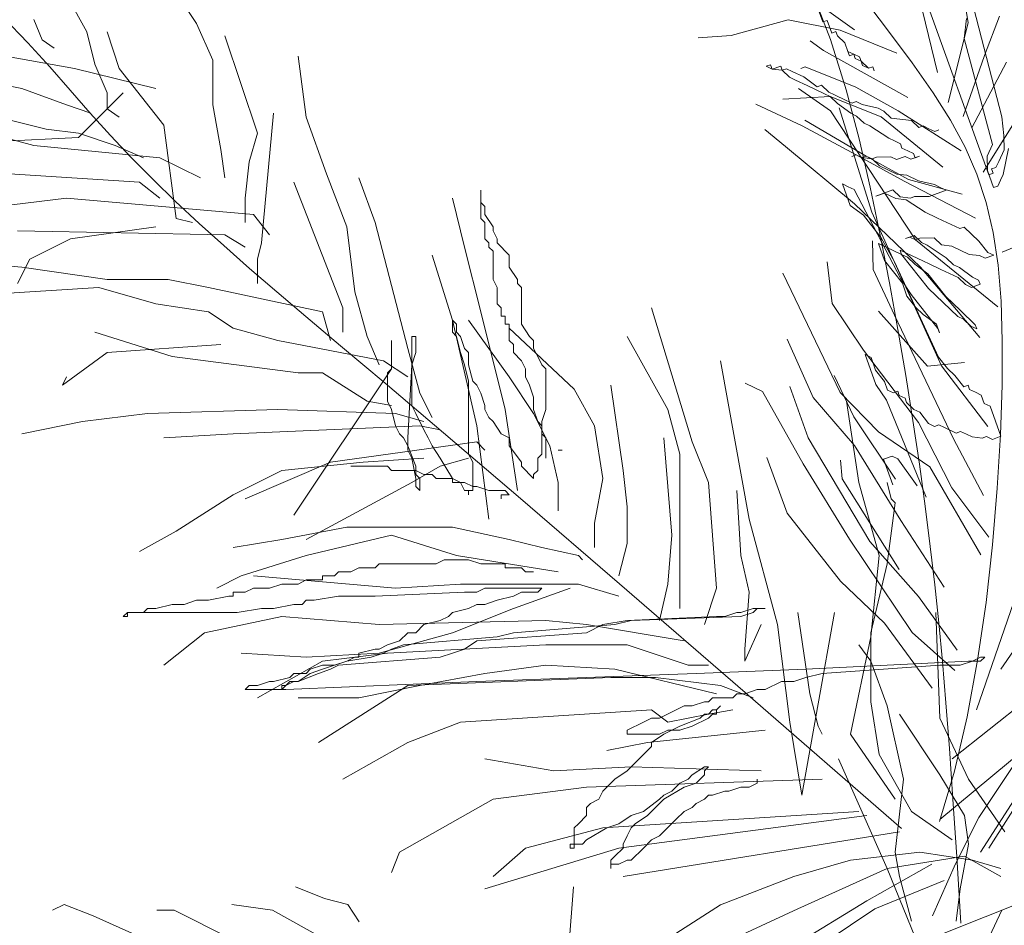
# Model space of a CAD drawing. Units: millimetres. Extents: x 595116 to 630915, y 909473 to 920225.
# Tile 87 of 134: x 629714.705 to 629720.901, y 919275.684 to 919281.384. Entities that reach past the tile are written whole.
import ezdxf

# ---------------------------------------------------------------- set-up
doc = ezdxf.new("R2010")
doc.units = ezdxf.units.MM
doc.layers.add('Dimension', color=3, linetype='Continuous', lineweight=18)
doc.layers.add('L-PLNT', color=85, linetype='Continuous', lineweight=13)
doc.styles.get("Standard").update_dxf_attribs({"font": 'arial.ttf'})
doc.dimstyles.new('ISO-25', dxfattribs={"dimtxt": 9, "dimasz": 6, "dimexe": 1.25, "dimexo": 0.625, "dimtad": 1, "dimlunit": 4, "dimtxsty": 'Standard', "dimcen": 2.5, "dimadec": 0, "dimazin": 0, "dimtfac": 1, "dimtmove": 0, "dimatfit": 3, "dimfxl": 1, "dimarcsym": 0})

# ---------------------------------------------------------------- blocks, each defined once
blk = doc.blocks.new('A$C4FB75ABC')
for p, q in [((2.7169, 3.7399), (2.6018, 4.2172)), ((2.8029, 3.5683), (2.5783, 4.1926)), ((1.2153, 3.9442), (1.2902, 3.808)), ((1.3924, 3.9442), (1.4742, 3.8217)), ((2.7679, 3.8231), (2.7507, 3.9385)), ((2.7636, 3.9026), (2.8247, 3.6653)), ((2.5777, 3.8114), (2.4796, 3.8815)), ((2.5372, 3.7949), (2.5035, 3.8821)), ((2.5794, 3.8826), (2.6314, 3.8136)), ((1.1917, 3.7897), (1.1506, 3.8319)), ((2.5166, 3.8462), (2.5244, 3.8247)), ((2.7613, 3.7965), (2.7653, 3.8303)), ((2.7957, 3.7683), (2.8207, 3.834)), ((1.2017, 3.8285), (1.2153, 3.7944)), ((1.4742, 3.8217), (1.5014, 3.7604)), ((2.4664, 3.8281), (2.3706, 3.8017)), ((2.5536, 3.8109), (2.4664, 3.8281)), ((2.5244, 3.8247), (2.5315, 3.8272)), ((2.5315, 3.8272), (2.5393, 3.8057)), ((2.7349, 3.6897), (2.7679, 3.8231)), ((1.2902, 3.808), (1.3039, 3.7536)), ((1.3243, 3.808), (1.3447, 3.7467)), ((1.5219, 3.8012), (1.5764, 3.6378)), ((2.3706, 3.8017), (2.3152, 3.798)), ((2.5393, 3.8057), (2.5464, 3.8083)), ((2.5464, 3.8083), (2.549, 3.8011)), ((2.549, 3.8011), (2.5614, 3.7893)), ((2.6486, 3.7721), (2.5536, 3.8109)), ((2.6314, 3.8136), (2.6743, 3.7558)), ((1.0382, 3.7876), (1.2698, 3.7467)), ((1.2284, 3.7492), (1.1917, 3.7897)), ((1.2153, 3.7944), (1.2357, 3.7808)), ((2.5255, 3.7764), (2.5034, 3.7928)), ((2.5638, 3.7106), (2.5372, 3.7949)), ((2.5614, 3.7893), (2.5665, 3.775)), ((2.8089, 3.6191), (2.7613, 3.7965)), ((1.6445, 3.7672), (1.6581, 3.665)), ((2.6672, 3.6978), (2.5255, 3.7764)), ((2.5665, 3.775), (2.5763, 3.7704)), ((2.5691, 3.7678), (2.5665, 3.775)), ((2.5763, 3.7704), (2.5691, 3.7678)), ((2.5763, 3.7704), (2.5789, 3.7632)), ((2.586, 3.7658), (2.5763, 3.7704)), ((2.5886, 3.7586), (2.586, 3.7658)), ((2.7596, 3.6662), (2.7957, 3.7683)), ((1.2625, 3.7099), (1.2284, 3.7492)), ((1.3039, 3.7536), (1.3243, 3.7059)), ((1.5014, 3.7604), (1.5014, 3.6855)), ((2.4369, 3.7526), (2.4297, 3.7501)), ((2.4297, 3.7501), (2.4394, 3.7455)), ((2.4394, 3.7455), (2.4369, 3.7526)), ((2.4538, 3.7506), (2.4394, 3.7455)), ((2.4564, 3.7435), (2.4538, 3.7506)), ((2.4948, 3.7492), (2.4876, 3.7466)), ((2.58, 3.715), (2.4948, 3.7492)), ((2.5789, 3.7632), (2.5886, 3.7586)), ((2.5886, 3.7586), (2.5912, 3.7515)), ((2.601, 3.7469), (2.5886, 3.7586)), ((2.5912, 3.7515), (2.601, 3.7469)), ((2.601, 3.7469), (2.6081, 3.7494)), ((2.6081, 3.7494), (2.601, 3.7469)), ((2.6081, 3.7494), (2.6107, 3.7423)), ((2.6107, 3.7423), (2.6081, 3.7494)), ((2.6743, 3.7558), (2.7096, 3.7056)), ((2.7745, 3.6472), (2.8322, 3.7571)), ((1.079, 3.7331), (1.1812, 3.7127)), ((1.2698, 3.7467), (1.4061, 3.7127)), ((1.3447, 3.7467), (1.4197, 3.6514)), ((2.4394, 3.7455), (2.4564, 3.7435)), ((2.4635, 3.746), (2.4564, 3.7435)), ((2.4564, 3.7435), (2.4687, 3.7317)), ((2.4733, 3.7414), (2.4635, 3.746)), ((2.4687, 3.7317), (2.4785, 3.7271)), ((2.4928, 3.7323), (2.4733, 3.7414)), ((2.5149, 3.7159), (2.4928, 3.7323)), ((2.4785, 3.7271), (2.498, 3.7179)), ((2.498, 3.7179), (2.5272, 3.7041)), ((2.5221, 3.7185), (2.5149, 3.7159)), ((2.5344, 3.7067), (2.5221, 3.7185)), ((2.6509, 3.6757), (2.58, 3.715)), ((1.1812, 3.7127), (1.2562, 3.6855)), ((1.2959, 3.6716), (1.2625, 3.7099)), ((1.3515, 3.7059), (1.2766, 3.631)), ((1.3243, 3.7059), (1.3243, 3.6787)), ((2.537, 3.6995), (2.4575, 3.6952)), ((2.5376, 3.6754), (2.4836, 3.7127)), ((2.5272, 3.7041), (2.537, 3.6995)), ((2.5441, 3.7021), (2.5344, 3.7067)), ((2.537, 3.6995), (2.5493, 3.6877)), ((2.6222, 3.6653), (2.537, 3.6995)), ((2.5637, 3.6929), (2.5441, 3.7021)), ((2.5853, 3.6284), (2.5638, 3.7106)), ((2.7096, 3.7056), (2.7388, 3.6597)), ((1.2562, 3.6855), (1.297, 3.6718)), ((1.5014, 3.6855), (1.5151, 3.6106)), ((2.4899, 3.6502), (2.4119, 3.6869)), ((2.5493, 3.6877), (2.5714, 3.6714)), ((2.5734, 3.6883), (2.5637, 3.6929)), ((2.5806, 3.6909), (2.5734, 3.6883)), ((2.5903, 3.6863), (2.5806, 3.6909)), ((2.617, 3.6797), (2.5903, 3.6863)), ((2.7932, 3.5729), (2.8652, 3.6879)), ((1.3299, 3.6341), (1.2959, 3.6716)), ((1.3243, 3.6787), (1.3447, 3.665)), ((1.6036, 3.6718), (1.5832, 3.4539)), ((2.6801, 3.4593), (2.5376, 3.6754)), ((2.6067, 3.5058), (2.5519, 3.6806)), ((2.5714, 3.6714), (2.5812, 3.6668)), ((2.5812, 3.6668), (2.5935, 3.655)), ((2.6268, 3.6751), (2.617, 3.6797)), ((2.7255, 3.5809), (2.6222, 3.6653)), ((2.6391, 3.6633), (2.6268, 3.6751)), ((2.7562, 3.6082), (2.6509, 3.6757)), ((2.8247, 3.6653), (2.8279, 3.634)), ((1.1403, 3.665), (1.2221, 3.6446)), ((1.4197, 3.6514), (1.4401, 3.4948)), ((1.6581, 3.665), (1.6922, 3.5697)), ((2.5803, 3.6016), (2.4899, 3.6502)), ((2.5972, 3.5996), (2.4945, 3.6599)), ((2.5935, 3.655), (2.6032, 3.6504)), ((2.6032, 3.6504), (2.6351, 3.6295)), ((2.673, 3.6593), (2.6391, 3.6633)), ((2.6853, 3.6475), (2.673, 3.6593)), ((2.6925, 3.6501), (2.6853, 3.6475)), ((2.7022, 3.6455), (2.6925, 3.6501)), ((2.7388, 3.6597), (2.763, 3.6147)), ((1.1267, 3.6378), (1.2017, 3.6174)), ((1.2221, 3.6446), (1.2766, 3.6378)), ((1.2766, 3.6378), (1.3379, 3.6174)), ((1.365, 3.5971), (1.3299, 3.6341)), ((1.5764, 3.6378), (1.5627, 3.5901)), ((2.4618, 3.6157), (2.4274, 3.6439)), ((2.712, 3.6409), (2.7022, 3.6455)), ((2.7192, 3.6435), (2.712, 3.6409)), ((2.8279, 3.634), (2.8285, 3.6099)), ((1.2766, 3.631), (1.1403, 3.6242)), ((1.2017, 3.6174), (1.4129, 3.5969)), ((1.3379, 3.6174), (1.3856, 3.5969)), ((2.5774, 3.5196), (2.4618, 3.6157)), ((2.6037, 3.5475), (2.5853, 3.6284)), ((2.6351, 3.6295), (2.6448, 3.6249)), ((2.6448, 3.6249), (2.6546, 3.6203)), ((2.6546, 3.6203), (2.6572, 3.6131)), ((2.7998, 3.5996), (2.8089, 3.6191)), ((1.5151, 3.6106), (1.5219, 3.5629)), ((2.5803, 3.6016), (2.5731, 3.5991)), ((2.5731, 3.5991), (2.5803, 3.6016)), ((2.5901, 3.597), (2.5803, 3.6016)), ((2.5803, 3.6016), (2.5901, 3.597)), ((2.6609, 3.5577), (2.5803, 3.6016)), ((2.5972, 3.5996), (2.5901, 3.597)), ((2.607, 3.595), (2.5972, 3.5996)), ((2.6681, 3.5603), (2.5972, 3.5996)), ((2.6572, 3.6131), (2.6669, 3.6085)), ((2.6669, 3.6085), (2.6767, 3.6039)), ((2.6864, 3.5993), (2.6721, 3.5942)), ((2.6767, 3.6039), (2.6793, 3.5967)), ((2.6793, 3.5967), (2.6864, 3.5993)), ((2.763, 3.6147), (2.7827, 3.5691)), ((2.8003, 3.5755), (2.7998, 3.5996)), ((2.8285, 3.6099), (2.8193, 3.5904)), ((2.8356, 3.6125), (2.827, 3.5688)), ((1.4014, 3.5604), (1.365, 3.5971)), ((1.4129, 3.5969), (1.481, 3.5629)), ((1.5627, 3.5901), (1.5559, 3.5288)), ((2.5901, 3.597), (2.607, 3.595)), ((2.6142, 3.5976), (2.607, 3.595)), ((2.607, 3.595), (2.6193, 3.5833)), ((2.6383, 3.5982), (2.6142, 3.5976)), ((2.6193, 3.5833), (2.6486, 3.5695)), ((2.648, 3.5936), (2.6383, 3.5982)), ((2.6623, 3.5987), (2.648, 3.5936)), ((2.6721, 3.5942), (2.6623, 3.5987)), ((2.8193, 3.5904), (2.8147, 3.5806)), ((1.1608, 3.5697), (1.3788, 3.5561)), ((1.6922, 3.5697), (1.7263, 3.4812)), ((2.6486, 3.5695), (2.6655, 3.5675)), ((2.6655, 3.5675), (2.685, 3.5583)), ((2.7827, 3.5691), (2.7983, 3.5216)), ((2.8107, 3.5468), (2.8003, 3.5755)), ((2.8101, 3.5709), (2.8029, 3.5683)), ((2.8147, 3.5806), (2.8075, 3.578)), ((2.8075, 3.578), (2.8101, 3.5709)), ((2.827, 3.5688), (2.8224, 3.5591)), ((1.3788, 3.5561), (1.4129, 3.5288)), ((1.4393, 3.5237), (1.4014, 3.5604)), ((1.6377, 3.5561), (1.7194, 3.345)), ((1.7467, 3.5629), (1.7739, 3.488)), ((2.5671, 3.5483), (2.5573, 3.5529)), ((2.5573, 3.5529), (2.5703, 3.517)), ((2.7805, 3.4954), (2.6609, 3.5577)), ((2.7579, 3.5359), (2.6681, 3.5603)), ((2.685, 3.5583), (2.7117, 3.5517)), ((2.7117, 3.5517), (2.7214, 3.5471)), ((2.8224, 3.5591), (2.8178, 3.5493)), ((1.9511, 3.4948), (1.9511, 3.5425)), ((1.9511, 3.5425), (1.9511, 3.522)), ((2.5769, 3.5437), (2.5671, 3.5483)), ((2.6552, 3.3935), (2.5769, 3.5437)), ((2.6204, 3.467), (2.6037, 3.5475)), ((2.642, 3.5428), (2.6133, 3.5325)), ((2.6133, 3.5325), (2.6276, 3.5376)), ((2.6276, 3.5376), (2.6471, 3.5284)), ((2.6543, 3.531), (2.642, 3.5428)), ((2.7312, 3.5425), (2.7025, 3.5321)), ((2.7214, 3.5471), (2.7312, 3.5425)), ((2.8178, 3.5493), (2.8107, 3.5468)), ((1.0858, 3.5084), (1.2562, 3.5288)), ((1.2562, 3.5288), (1.5696, 3.5016)), ((1.4788, 3.4868), (1.4393, 3.5237)), ((1.5559, 3.5288), (1.5559, 3.488)), ((1.9034, 3.5288), (1.9238, 3.4471)), ((1.9511, 3.522), (1.9579, 3.5152)), ((2.5703, 3.517), (2.5924, 3.5006)), ((2.6885, 3.4136), (2.5774, 3.5196)), ((2.6471, 3.5284), (2.6641, 3.5264)), ((2.6712, 3.529), (2.6543, 3.531)), ((2.6641, 3.5264), (2.6959, 3.5055)), ((2.6784, 3.5316), (2.6712, 3.529)), ((2.7025, 3.5321), (2.6784, 3.5316)), ((2.7983, 3.5216), (2.81, 3.4712)), ((1.5696, 3.5016), (1.5968, 3.4676)), ((1.9579, 3.5152), (1.9579, 3.5016)), ((1.9579, 3.5016), (1.9715, 3.4812)), ((2.5924, 3.5006), (2.6222, 3.4627)), ((2.7237, 3.248), (2.6067, 3.5058)), ((2.6959, 3.5055), (2.7154, 3.4963)), ((1.4401, 3.4948), (1.4674, 3.488)), ((1.5201, 3.4494), (1.4788, 3.4868)), ((1.7739, 3.488), (1.8285, 3.2769)), ((1.9579, 3.488), (1.9511, 3.4948)), ((1.9579, 3.4608), (1.9579, 3.488)), ((2.7154, 3.4963), (2.7252, 3.4917)), ((2.7252, 3.4917), (2.7544, 3.4779)), ((2.8253, 3.4385), (2.9518, 3.4922)), ((1.1744, 3.4744), (1.5219, 3.4676)), ((1.4061, 3.4812), (1.263, 3.4608)), ((1.5219, 3.4676), (1.5559, 3.4471)), ((1.7263, 3.4812), (1.7399, 3.3722)), ((1.9715, 3.4812), (1.9715, 3.4744)), ((1.9715, 3.4744), (1.9783, 3.4608)), ((2.636, 3.3873), (2.6204, 3.467)), ((2.7544, 3.4779), (2.7616, 3.4805)), ((2.7616, 3.4805), (2.774, 3.4687)), ((2.774, 3.4687), (2.7863, 3.4569)), ((2.81, 3.4712), (2.8183, 3.4166)), ((1.263, 3.4608), (1.1949, 3.4267)), ((1.5832, 3.4539), (1.5764, 3.4267)), ((1.9647, 3.4539), (1.9579, 3.4608)), ((1.9647, 3.4471), (1.9647, 3.4539)), ((1.9783, 3.4608), (1.9783, 3.4539)), ((1.9783, 3.4539), (1.9988, 3.4335)), ((2.609, 3.4093), (2.6078, 3.4576)), ((2.6566, 3.4346), (2.6176, 3.453)), ((2.6176, 3.453), (2.6279, 3.4243)), ((2.6222, 3.4627), (2.6449, 3.4222)), ((2.6632, 3.4613), (2.6776, 3.4664)), ((2.6704, 3.4639), (2.6632, 3.4613)), ((2.6801, 3.4593), (2.6704, 3.4639)), ((2.6776, 3.4664), (2.6899, 3.4547)), ((2.6873, 3.4618), (2.6801, 3.4593)), ((2.8178, 3.3467), (2.6801, 3.4593)), ((2.7114, 3.4624), (2.6873, 3.4618)), ((2.6899, 3.4547), (2.6996, 3.4501)), ((2.7237, 3.4506), (2.7114, 3.4624)), ((2.7407, 3.4486), (2.7237, 3.4506)), ((2.7863, 3.4569), (2.8012, 3.438)), ((1.5633, 3.4112), (1.5201, 3.4494)), ((1.9238, 3.4471), (1.9511, 3.3382)), ((1.9715, 3.4403), (1.9647, 3.4471)), ((1.9715, 3.3927), (1.9715, 3.4403)), ((2.6638, 3.4372), (2.654, 3.4418)), ((2.654, 3.4418), (2.6566, 3.4346)), ((2.6566, 3.4346), (2.6664, 3.43)), ((2.6865, 3.3967), (2.6566, 3.4346)), ((2.693, 3.4234), (2.6638, 3.4372)), ((2.6996, 3.4501), (2.7315, 3.4291)), ((2.7699, 3.4348), (2.7407, 3.4486)), ((2.7869, 3.4328), (2.7699, 3.4348)), ((2.8012, 3.438), (2.811, 3.4334)), ((1.0245, 3.4267), (1.1812, 3.4131)), ((1.1949, 3.4267), (1.1744, 3.3858)), ((1.5764, 3.4267), (1.5764, 3.3858)), ((1.8693, 3.4335), (1.9034, 3.3246)), ((1.9988, 3.4335), (1.9988, 3.4131)), ((2.5404, 3.3522), (2.5315, 3.422)), ((2.6279, 3.4243), (2.6578, 3.3864)), ((2.6449, 3.4222), (2.7186, 3.2624)), ((2.6664, 3.43), (2.6787, 3.4182)), ((2.6787, 3.4182), (2.7008, 3.4019)), ((2.7028, 3.4188), (2.693, 3.4234)), ((2.7223, 3.4096), (2.7028, 3.4188)), ((2.7315, 3.4291), (2.7438, 3.4173)), ((2.7966, 3.4282), (2.7869, 3.4328)), ((2.811, 3.4334), (2.7966, 3.4282)), ((1.1812, 3.4131), (1.3243, 3.3927)), ((1.6088, 3.3721), (1.5633, 3.4112)), ((1.9988, 3.4131), (2.0124, 3.3927)), ((2.5536, 3.203), (2.4572, 3.4034)), ((2.6446, 3.333), (2.609, 3.4093)), ((2.7877, 3.2953), (2.6885, 3.4136)), ((2.7008, 3.4019), (2.7306, 3.364)), ((2.7516, 3.3958), (2.7223, 3.4096)), ((2.7438, 3.4173), (2.7536, 3.4127)), ((2.7536, 3.4127), (2.7757, 3.3964)), ((2.8183, 3.4166), (2.8233, 3.3565)), ((1.3243, 3.3927), (1.4265, 3.3927)), ((1.4265, 3.3927), (1.4946, 3.379)), ((1.9783, 3.379), (1.9715, 3.3927)), ((2.0124, 3.3927), (2.0124, 3.3858)), ((2.0124, 3.3858), (2.0192, 3.379)), ((2.6503, 3.3086), (2.636, 3.3873)), ((2.6727, 3.3674), (2.6552, 3.3935)), ((2.6578, 3.3864), (2.6655, 3.3648)), ((2.7014, 3.3777), (2.6865, 3.3967)), ((2.7639, 3.384), (2.7516, 3.3958)), ((2.788, 3.3846), (2.7737, 3.3794)), ((2.7757, 3.3964), (2.7854, 3.3918)), ((2.7854, 3.3918), (2.788, 3.3846)), ((0.9768, 3.3586), (1.3107, 3.379)), ((1.3107, 3.379), (1.4061, 3.3518)), ((1.4946, 3.379), (1.6854, 3.3382)), ((1.6577, 3.3307), (1.6088, 3.3721)), ((1.7399, 3.3722), (1.7603, 3.2973)), ((1.9783, 3.3518), (1.9783, 3.379)), ((2.0192, 3.379), (2.0192, 3.3178)), ((2.7384, 3.3424), (2.7014, 3.3777)), ((2.7737, 3.3794), (2.7639, 3.384)), ((1.4061, 3.3518), (1.4946, 3.3382)), ((1.9851, 3.345), (1.9783, 3.3518)), ((2.5929, 3.2739), (2.5404, 3.3522)), ((2.6655, 3.3648), (2.6804, 3.3459)), ((2.7174, 3.3106), (2.6727, 3.3674)), ((2.7306, 3.364), (2.743, 3.3522)), ((2.743, 3.3522), (2.7553, 3.3404)), ((2.8233, 3.3565), (2.8254, 3.2898)), ((1.4946, 3.3382), (1.5355, 3.3109)), ((1.6854, 3.3382), (1.699, 3.2905)), ((1.7194, 3.345), (1.7194, 3.3041)), ((1.9511, 3.3382), (1.992, 3.1748)), ((1.9851, 3.3314), (1.9851, 3.345)), ((2.2372, 3.345), (2.3054, 3.1203)), ((2.6997, 3.2474), (2.6179, 3.3396)), ((2.6804, 3.3459), (2.6928, 3.3341)), ((2.7507, 3.3307), (2.7384, 3.3424)), ((2.7553, 3.3404), (2.78, 3.3169)), ((1.7159, 3.2817), (1.6577, 3.3307)), ((1.9102, 3.3178), (1.9034, 3.3246)), ((1.9034, 3.3246), (1.9034, 3.3041)), ((1.9034, 3.3246), (1.9443, 3.1475)), ((1.9306, 3.3246), (1.9988, 3.2292)), ((1.992, 3.3314), (1.9851, 3.3314)), ((1.992, 3.3178), (1.992, 3.3314)), ((2.7435, 3.1255), (2.6446, 3.333)), ((2.6928, 3.3341), (2.7149, 3.3178)), ((2.7605, 3.3261), (2.7507, 3.3307)), ((2.7728, 3.3143), (2.7605, 3.3261)), ((1.3039, 3.3041), (1.4333, 3.2633)), ((1.5355, 3.3109), (1.6104, 3.2905)), ((1.9034, 3.3041), (1.9102, 3.2973)), ((1.9102, 3.3041), (1.9102, 3.3178)), ((1.917, 3.2973), (1.9102, 3.3041)), ((1.9988, 3.3178), (1.992, 3.3178)), ((1.9988, 3.2905), (1.9988, 3.3178)), ((1.9988, 3.3109), (2.1078, 3.2088)), ((2.0192, 3.3178), (2.0328, 3.2973)), ((2.6635, 3.2315), (2.6503, 3.3086)), ((2.7149, 3.3178), (2.72, 3.3034)), ((2.72, 3.3034), (2.7174, 3.3106)), ((2.7826, 3.3097), (2.7728, 3.3143)), ((2.78, 3.3169), (2.7826, 3.3097)), ((1.6104, 3.2905), (1.7876, 3.2565)), ((1.7603, 3.2973), (1.7808, 3.2497)), ((1.8012, 3.2429), (1.8012, 3.2905)), ((1.8012, 3.2905), (1.8012, 3.2429)), ((1.8421, 3.2973), (1.8353, 3.2973)), ((1.8353, 3.2973), (1.8353, 3.2497)), ((1.8421, 3.2701), (1.8421, 3.2973)), ((1.9102, 3.2973), (1.917, 3.2701)), ((1.9238, 3.2769), (1.917, 3.2973)), ((2.0056, 3.2837), (1.9988, 3.2905)), ((2.0328, 3.2973), (2.0396, 3.2905)), ((2.0396, 3.2905), (2.0396, 3.2769)), ((2.1963, 3.2973), (2.2645, 3.1748)), ((2.508, 3.1947), (2.4647, 3.2926)), ((2.8254, 3.2898), (2.825, 3.2153)), ((1.3243, 3.2701), (1.2494, 3.2156)), ((1.5151, 3.2837), (1.3243, 3.2701)), ((1.7906, 3.2188), (1.7159, 3.2817)), ((1.8285, 3.2769), (1.8489, 3.202)), ((1.8353, 3.2497), (1.8421, 3.2701)), ((1.917, 3.2701), (1.9238, 3.2497)), ((1.9306, 3.2701), (1.9238, 3.2769)), ((1.9306, 3.2497), (1.9306, 3.2701)), ((2.0056, 3.2701), (2.0056, 3.2837)), ((2.0192, 3.2565), (2.0056, 3.2701)), ((2.0396, 3.2769), (2.0465, 3.2633)), ((2.685, 3.153), (2.5929, 3.2739)), ((1.4333, 3.2633), (1.6445, 3.236)), ((1.7876, 3.2565), (1.8285, 3.2292)), ((2.026, 3.2429), (2.0192, 3.2565)), ((2.0465, 3.2633), (2.0533, 3.2497)), ((2.353, 3.2565), (2.4007, 2.9909)), ((2.6053, 3.2621), (2.5955, 3.2667)), ((2.5955, 3.2667), (2.6136, 3.2165)), ((2.613, 3.2406), (2.6053, 3.2621)), ((2.7622, 3.2537), (2.6997, 3.2474)), ((2.7186, 3.2624), (2.7335, 3.2434)), ((1.8012, 3.2429), (1.6377, 2.9977)), ((1.6445, 3.236), (1.6854, 3.236)), ((1.6854, 3.236), (1.7603, 3.1884)), ((1.7944, 3.236), (1.8012, 3.2429)), ((1.7944, 3.1884), (1.7944, 3.236)), ((1.8353, 3.2497), (1.8285, 3.1271)), ((1.8353, 3.1816), (1.8353, 3.2497)), ((1.9238, 3.2497), (1.9306, 3.2224)), ((1.9375, 3.2224), (1.9306, 3.2497)), ((2.026, 3.2292), (2.026, 3.2429)), ((2.0533, 3.2497), (2.0601, 3.2429)), ((2.0601, 3.2429), (2.0601, 3.1748)), ((2.6279, 3.2216), (2.613, 3.2406)), ((2.8009, 3.1461), (2.7237, 3.248)), ((2.7335, 3.2434), (2.7458, 3.2316)), ((1.2494, 3.2156), (1.2562, 3.2292)), ((1.9306, 3.2224), (1.9306, 3.0999)), ((1.9443, 3.2156), (1.9375, 3.2224)), ((1.9988, 3.2292), (2.0396, 3.1679)), ((2.0328, 3.2156), (2.026, 3.2292)), ((2.5763, 3.1625), (2.5433, 3.2317)), ((2.6331, 3.2073), (2.6279, 3.2216)), ((2.6754, 3.1561), (2.6635, 3.2315)), ((2.7458, 3.2316), (2.7608, 3.2127)), ((1.8887, 3.1355), (1.7906, 3.2188)), ((1.9511, 3.202), (1.9443, 3.2156)), ((2.0396, 3.1952), (2.0328, 3.2156)), ((2.1078, 3.2088), (2.1418, 3.1475)), ((2.1691, 3.2156), (2.1895, 3.0726)), ((2.4234, 3.2048), (2.3941, 3.2186)), ((2.4914, 3.0833), (2.4234, 3.2048)), ((2.5, 3.127), (2.469, 3.2131)), ((2.6179, 3.137), (2.5536, 3.203)), ((2.6136, 3.2165), (2.6311, 3.1904)), ((2.6428, 3.2027), (2.6331, 3.2073)), ((2.65, 3.2053), (2.6428, 3.2027)), ((2.6526, 3.1981), (2.65, 3.2053)), ((2.7608, 3.2127), (2.7679, 3.2153)), ((2.7679, 3.2153), (2.7705, 3.2081)), ((2.7705, 3.2081), (2.7803, 3.2035)), ((2.7803, 3.2035), (2.79, 3.1989)), ((2.825, 3.2153), (2.8223, 3.1323)), ((1.7603, 3.1884), (1.8012, 3.1816)), ((1.8012, 3.1748), (1.7944, 3.1884)), ((1.8489, 3.202), (1.8693, 3.1611)), ((1.9579, 3.1816), (1.9511, 3.202)), ((2.0396, 3.1748), (2.0396, 3.1952)), ((2.5774, 3.1143), (2.508, 3.1947)), ((2.5847, 3.0522), (2.5642, 3.1884)), ((2.6311, 3.1904), (2.6976, 3.0279)), ((2.6624, 3.1935), (2.6526, 3.1981)), ((2.6649, 3.1863), (2.6624, 3.1935)), ((2.6773, 3.1746), (2.6649, 3.1863)), ((2.79, 3.1989), (2.7952, 3.1846)), ((1.3924, 3.1679), (1.6104, 3.1748)), ((1.6104, 3.1748), (1.808, 3.1679)), ((1.808, 3.1475), (1.8012, 3.1748)), ((1.8421, 3.1679), (1.8353, 3.1816)), ((1.9579, 3.1748), (1.9579, 3.1816)), ((1.9647, 3.1611), (1.9579, 3.1748)), ((1.992, 3.1748), (2.0124, 3.0386)), ((2.0465, 3.1543), (2.0396, 3.1748)), ((2.0601, 3.1748), (2.0533, 3.1543)), ((2.2645, 3.1748), (2.2849, 3.0999)), ((2.687, 3.17), (2.6773, 3.1746)), ((2.7019, 3.151), (2.687, 3.17)), ((2.7952, 3.1846), (2.8049, 3.18)), ((2.8049, 3.18), (2.823, 3.1297)), ((1.1812, 3.1339), (1.2834, 3.1543)), ((1.2834, 3.1543), (1.3924, 3.1679)), ((1.808, 3.1679), (1.8557, 3.1543)), ((1.8557, 3.1407), (1.8421, 3.1679)), ((1.9715, 3.1543), (1.9647, 3.1611)), ((1.9851, 3.1339), (1.9715, 3.1543)), ((2.0396, 3.1679), (2.0669, 3.1135)), ((2.0533, 3.1475), (2.0465, 3.1543)), ((2.0533, 3.1543), (2.0533, 3.0999)), ((2.6463, 3.058), (2.5763, 3.1625)), ((2.6863, 3.0831), (2.6754, 3.1561)), ((1.5355, 3.1339), (1.8489, 3.1475)), ((1.8148, 3.1339), (1.808, 3.1475)), ((1.8489, 3.1475), (1.883, 3.1407)), ((1.8625, 3.1271), (1.8557, 3.1407)), ((1.9443, 3.1475), (1.9647, 2.9909)), ((2.0533, 3.1339), (2.0533, 3.1475)), ((2.1418, 3.1475), (2.1555, 3.059)), ((2.7037, 3.0787), (2.6179, 3.137)), ((2.7407, 3.0434), (2.685, 3.153)), ((2.7117, 3.1464), (2.7019, 3.151)), ((2.7189, 3.149), (2.7117, 3.1464)), ((2.7286, 3.1444), (2.7189, 3.149)), ((2.7481, 3.1352), (2.7286, 3.1444)), ((2.7553, 3.1378), (2.7481, 3.1352)), ((2.7651, 3.1332), (2.7553, 3.1378)), ((1.4197, 3.1271), (1.5355, 3.1339)), ((1.699, 3.0862), (1.9443, 3.1203)), ((1.8216, 3.1271), (1.8148, 3.1339)), ((1.8285, 3.1135), (1.8216, 3.1271)), ((1.8285, 3.1271), (1.8285, 3.1067)), ((1.8693, 3.1135), (1.8625, 3.1271)), ((2.0174, 3.0255), (1.8887, 3.1355)), ((1.9443, 3.1203), (1.9579, 3.1067)), ((1.9988, 3.1271), (1.9851, 3.1339)), ((1.9988, 3.1135), (1.9988, 3.1271)), ((2.0601, 3.1271), (2.0533, 3.1339)), ((2.0601, 3.093), (2.0601, 3.1271)), ((2.2577, 3.1271), (2.2713, 2.9637)), ((2.3054, 3.1203), (2.3326, 3.0522)), ((2.603, 2.9533), (2.5, 3.127)), ((2.794, 3.0302), (2.7435, 3.1255)), ((2.7748, 3.1286), (2.7651, 3.1332)), ((2.7917, 3.1266), (2.7748, 3.1286)), ((2.7823, 2.6709), (2.9389, 3.1271)), ((2.7989, 3.1292), (2.7917, 3.1266)), ((2.8087, 3.1246), (2.7989, 3.1292)), ((2.823, 3.1297), (2.8087, 3.1246)), ((2.8223, 3.1323), (2.817, 3.0425)), ((1.8421, 3.0794), (1.8285, 3.1135)), ((1.8285, 3.1067), (1.8353, 3.093)), ((1.883, 3.093), (1.8693, 3.1135)), ((2.0192, 3.0862), (1.9988, 3.1135)), ((2.0669, 3.1135), (2.0805, 3.0522)), ((2.0873, 3.1067), (2.0805, 3.1067)), ((2.6552, 2.9883), (2.5774, 3.1143)), ((1.8557, 3.093), (1.7535, 3.0862)), ((1.8353, 3.093), (1.8421, 3.059)), ((1.9034, 3.059), (1.883, 3.093)), ((1.883, 3.0794), (1.9306, 3.093)), ((1.9306, 3.0999), (1.9375, 3.0862)), ((2.0533, 3.0999), (2.0465, 3.093)), ((2.0465, 3.093), (2.0465, 3.0726)), ((2.2849, 3.0999), (2.2849, 2.9024)), ((2.4644, 3.0007), (2.4308, 3.094)), ((2.5571, 3.0584), (2.5539, 3.0896)), ((2.6406, 3.0965), (2.6262, 3.0913)), ((2.6262, 3.0913), (2.6417, 3.0483)), ((2.6503, 3.0919), (2.6406, 3.0965)), ((2.6827, 3.0468), (2.6503, 3.0919)), ((1.6173, 3.0726), (1.5355, 3.0318)), ((1.5559, 3.0249), (1.699, 3.0862)), ((1.7535, 3.0862), (1.6173, 3.0726)), ((1.7331, 3.0794), (1.7944, 3.0794)), ((1.7944, 3.0794), (1.8012, 3.0726)), ((1.8012, 3.0726), (1.8421, 3.0726)), ((1.8353, 3.0522), (1.883, 3.0794)), ((1.8421, 3.0658), (1.8421, 3.0794)), ((1.8421, 3.0726), (1.8557, 3.0658)), ((1.9375, 3.0862), (1.9375, 3.0386)), ((2.0192, 3.0794), (2.0192, 3.0862)), ((2.0396, 3.059), (2.0192, 3.0794)), ((2.0465, 3.0726), (2.0396, 3.0658)), ((2.1895, 3.0726), (2.1963, 3.0113)), ((2.5691, 2.9573), (2.4914, 3.0833)), ((2.696, 3.0126), (2.6863, 3.0831)), ((2.7892, 2.9311), (2.7037, 3.0787)), ((1.8489, 3.059), (1.8421, 3.0658)), ((1.8421, 3.059), (1.8421, 3.0454)), ((1.8489, 3.0386), (1.8489, 3.059)), ((1.8557, 3.0658), (1.8693, 3.0658)), ((1.8693, 3.0658), (1.8761, 3.059)), ((1.8761, 3.059), (1.9034, 3.059)), ((1.917, 3.0522), (1.9034, 3.059)), ((1.9034, 3.059), (1.9034, 3.0522)), ((2.0396, 3.0658), (2.0396, 3.059)), ((2.1555, 3.059), (2.1418, 2.9841)), ((2.6523, 2.9062), (2.5571, 3.0584)), ((1.6581, 2.9569), (1.8353, 3.0522)), ((1.8421, 3.0454), (1.8489, 3.0386)), ((1.9034, 3.0522), (1.9238, 3.0522)), ((1.9238, 3.0386), (1.917, 3.0522)), ((1.9238, 3.0522), (1.9375, 3.0454)), ((1.9306, 3.0386), (1.9238, 3.0386)), ((1.9375, 3.0386), (1.9306, 3.0386)), ((1.9306, 3.0386), (1.9306, 3.0318)), ((1.9306, 3.0318), (1.9306, 3.0386)), ((1.9375, 3.0454), (1.9443, 3.0454)), ((1.9443, 3.0454), (1.9647, 3.0386)), ((1.9647, 3.0386), (1.992, 3.0386)), ((1.992, 3.0386), (1.9988, 3.0318)), ((2.0805, 3.0522), (2.0805, 3.0045)), ((2.3326, 3.0522), (2.3462, 2.8751)), ((2.3803, 3.0386), (2.3871, 2.9296)), ((2.6187, 2.9296), (2.5847, 3.0522)), ((2.6392, 3.0249), (2.6324, 3.0522)), ((2.8029, 2.9604), (2.7407, 3.0434)), ((2.817, 3.0425), (2.809, 2.948)), ((1.5355, 3.0318), (1.4401, 2.9705)), ((1.9988, 3.0318), (1.9851, 3.0318)), ((1.9851, 3.0318), (1.9851, 3.0249)), ((2.1835, 2.8826), (2.0174, 3.0255)), ((2.646, 3.0181), (2.6392, 3.0249)), ((2.1963, 3.0113), (2.1963, 2.95)), ((2.6324, 2.916), (2.646, 3.0181)), ((2.7046, 2.9452), (2.696, 3.0126)), ((2.4007, 2.9909), (2.4484, 2.8139)), ((2.5539, 2.887), (2.4644, 3.0007)), ((2.7278, 2.8766), (2.6552, 2.9883)), ((1.6173, 2.9569), (1.7263, 2.9773)), ((1.7263, 2.9773), (1.9034, 2.9773)), ((1.9034, 2.9773), (1.9988, 2.9569)), ((2.1418, 2.9841), (2.1418, 2.9432)), ((1.4401, 2.9705), (1.3788, 2.9364)), ((1.5355, 2.9432), (1.6173, 2.9569)), ((1.8012, 2.9637), (1.6581, 2.9296)), ((1.9102, 2.9296), (1.8012, 2.9637)), ((1.9988, 2.9569), (2.0533, 2.9432)), ((2.2713, 2.9637), (2.2645, 2.882)), ((2.6741, 2.8006), (2.5691, 2.9573)), ((2.0533, 2.9432), (2.1146, 2.9296)), ((2.1963, 2.95), (2.1827, 2.8956)), ((2.6847, 2.8611), (2.603, 2.9533)), ((2.7122, 2.8807), (2.7046, 2.9452)), ((2.809, 2.948), (2.7981, 2.8512)), ((1.6581, 2.9296), (1.5491, 2.8956)), ((1.8898, 2.9228), (1.8761, 2.916)), ((1.9306, 2.9228), (1.8898, 2.9228)), ((2.0805, 2.9024), (1.9102, 2.9296)), ((1.9511, 2.916), (1.9306, 2.9228)), ((2.1146, 2.9296), (2.1214, 2.9228)), ((2.3871, 2.9296), (2.4007, 2.8683)), ((2.6051, 2.7934), (2.6187, 2.9296)), ((1.7467, 2.9092), (1.7331, 2.9024)), ((1.7739, 2.9092), (1.7467, 2.9092)), ((1.7808, 2.916), (1.7739, 2.9092)), ((1.8761, 2.916), (1.7808, 2.916)), ((1.992, 2.916), (1.9511, 2.916)), ((1.992, 2.9092), (1.992, 2.916)), ((2.0192, 2.9092), (1.992, 2.9092)), ((2.026, 2.9024), (2.0192, 2.9092)), ((2.6051, 2.8002), (2.6324, 2.916)), ((1.5491, 2.8956), (1.5082, 2.8751)), ((1.5696, 2.8956), (1.808, 2.8751)), ((1.6854, 2.8956), (1.6854, 2.8888)), ((1.7058, 2.8956), (1.6854, 2.8956)), ((1.7126, 2.9024), (1.7058, 2.8956)), ((1.7331, 2.9024), (1.7126, 2.9024)), ((2.0396, 2.9024), (2.026, 2.9024)), ((2.2849, 2.9024), (2.2849, 2.8411)), ((1.5696, 2.8751), (1.5559, 2.8683)), ((1.5968, 2.8751), (1.5696, 2.8751)), ((1.6173, 2.882), (1.5968, 2.8751)), ((1.6445, 2.882), (1.6173, 2.882)), ((1.6581, 2.8888), (1.6445, 2.882)), ((1.6854, 2.8888), (1.6581, 2.8888)), ((1.808, 2.8751), (1.917, 2.882)), ((1.917, 2.882), (2.1146, 2.882)), ((1.9443, 2.8683), (1.9579, 2.8751)), ((1.9579, 2.8751), (2.0533, 2.8751)), ((2.101, 2.8751), (2.0056, 2.8411)), ((2.0533, 2.8751), (2.0465, 2.8683)), ((2.1146, 2.882), (2.1827, 2.8615)), ((2.3943, 2.7002), (2.1835, 2.8826)), ((2.2645, 2.882), (2.2508, 2.8207)), ((2.3462, 2.8751), (2.3258, 2.8139)), ((2.6279, 2.8164), (2.5539, 2.887)), ((2.7189, 2.8171), (2.7122, 2.8807)), ((2.8231, 2.739), (2.9253, 2.8888)), ((1.5287, 2.8615), (1.4946, 2.8547)), ((1.5355, 2.8615), (1.5287, 2.8615)), ((1.5559, 2.8683), (1.5355, 2.8683)), ((1.5355, 2.8683), (1.5355, 2.8615)), ((1.6718, 2.8547), (1.7126, 2.8615)), ((1.7126, 2.8615), (1.7739, 2.8615)), ((1.7739, 2.8615), (1.9238, 2.8683)), ((1.9238, 2.8683), (1.9443, 2.8683)), ((2.0056, 2.8615), (1.9783, 2.8547)), ((2.0192, 2.8683), (2.0056, 2.8615)), ((2.0465, 2.8683), (2.0192, 2.8683)), ((2.4007, 2.8683), (2.3939, 2.773)), ((2.7496, 2.771), (2.6847, 2.8611)), ((1.3924, 2.8411), (1.3856, 2.8343)), ((1.4061, 2.8411), (1.3924, 2.8411)), ((1.4333, 2.8479), (1.4061, 2.8411)), ((1.4537, 2.8479), (1.4333, 2.8479)), ((1.4742, 2.8547), (1.4537, 2.8479)), ((1.4946, 2.8547), (1.4742, 2.8547)), ((1.5423, 2.8343), (1.5832, 2.8411)), ((1.5832, 2.8411), (1.6036, 2.8411)), ((1.6036, 2.8411), (1.6377, 2.8479)), ((1.6377, 2.8479), (1.6513, 2.8479)), ((1.6513, 2.8479), (1.6581, 2.8547)), ((1.6581, 2.8547), (1.6718, 2.8547)), ((1.9306, 2.8411), (1.9034, 2.8343)), ((2.0056, 2.8411), (1.9034, 2.8002)), ((1.9443, 2.8479), (1.9306, 2.8411)), ((1.9579, 2.8479), (1.9443, 2.8479)), ((1.9783, 2.8547), (1.9579, 2.8479)), ((2.3871, 2.8343), (2.4075, 2.8411)), ((2.4075, 2.8411), (2.428, 2.8411)), ((2.4144, 2.8411), (2.4075, 2.8343)), ((2.428, 2.8411), (2.4144, 2.8411)), ((2.7981, 2.8512), (2.784, 2.7542)), ((1.3515, 2.8275), (1.3584, 2.8343)), ((1.3584, 2.8275), (1.3515, 2.8275)), ((1.3856, 2.8343), (1.3584, 2.8343)), ((1.3584, 2.8343), (1.3584, 2.8275)), ((1.3584, 2.8343), (1.5423, 2.8343)), ((1.4878, 2.8002), (1.6173, 2.8275)), ((1.6173, 2.8275), (1.7808, 2.8139)), ((1.8966, 2.8275), (1.883, 2.8207)), ((1.9034, 2.8343), (1.8966, 2.8275)), ((2.1963, 2.8207), (2.3462, 2.8275)), ((2.3871, 2.8275), (2.2032, 2.8207)), ((2.3462, 2.8275), (2.3599, 2.8275)), ((2.3599, 2.8275), (2.3803, 2.8343)), ((2.3803, 2.8343), (2.3871, 2.8343)), ((2.4075, 2.8343), (2.3871, 2.8275)), ((2.4825, 2.8343), (2.5029, 2.6981)), ((2.4893, 2.5279), (2.5438, 2.8343)), ((2.7209, 2.6572), (2.7141, 2.8343)), ((1.7808, 2.8139), (2.0601, 2.8207)), ((1.8557, 2.8139), (1.8421, 2.8002)), ((1.883, 2.8207), (1.8557, 2.8139)), ((2.1759, 2.8139), (2.0056, 2.8002)), ((2.0601, 2.8207), (2.1282, 2.8139)), ((2.1282, 2.8002), (2.1555, 2.8139)), ((2.1282, 2.8139), (2.2917, 2.7866)), ((2.1555, 2.8139), (2.1963, 2.8207)), ((2.2032, 2.8207), (2.1759, 2.8139)), ((2.3939, 2.7526), (2.4212, 2.8139)), ((2.4484, 2.8139), (2.4689, 2.6504)), ((2.7077, 2.7073), (2.6279, 2.8164)), ((2.7251, 2.7519), (2.7189, 2.8171)), ((1.4197, 2.7458), (1.4878, 2.8002)), ((1.9034, 2.8002), (1.7808, 2.7662)), ((1.8285, 2.8002), (1.8148, 2.7866)), ((1.9783, 2.7934), (1.8216, 2.7798)), ((1.8421, 2.8002), (1.8285, 2.8002)), ((1.9443, 2.7866), (2.1282, 2.8002)), ((2.0056, 2.8002), (1.9783, 2.7934)), ((2.5711, 2.63), (2.6051, 2.7934)), ((2.6051, 2.6845), (2.6051, 2.8002)), ((2.7456, 2.7371), (2.6741, 2.8006)), ((1.7944, 2.7798), (1.7808, 2.773)), ((1.8148, 2.7866), (1.7944, 2.7798)), ((1.7944, 2.7662), (2.0601, 2.7798)), ((1.8216, 2.7798), (1.8012, 2.773)), ((1.9238, 2.773), (1.9443, 2.7866)), ((2.0601, 2.7798), (2.1078, 2.7798)), ((2.1078, 2.7798), (2.1963, 2.7798)), ((2.1963, 2.7798), (2.2985, 2.7458)), ((2.6051, 2.7526), (2.5847, 2.7798)), ((1.6581, 2.7594), (1.5491, 2.7662)), ((1.7808, 2.7662), (1.6581, 2.7594)), ((1.6854, 2.7526), (1.7944, 2.7662)), ((1.7126, 2.7458), (1.883, 2.7594)), ((1.7399, 2.7594), (1.7263, 2.7526)), ((1.7671, 2.7594), (1.7263, 2.7526)), ((1.7467, 2.7594), (1.7399, 2.7594)), ((1.7739, 2.773), (1.7467, 2.7662)), ((1.7467, 2.7662), (1.7467, 2.7594)), ((1.7876, 2.7662), (1.7671, 2.7594)), ((1.7808, 2.773), (1.7739, 2.773)), ((1.8012, 2.773), (1.7876, 2.7662)), ((1.883, 2.7594), (1.9034, 2.7662)), ((1.9034, 2.7662), (1.9238, 2.773)), ((2.3939, 2.773), (2.3939, 2.7526)), ((2.7891, 2.7594), (2.7754, 2.7526)), ((2.7891, 2.7526), (2.7959, 2.7594)), ((2.7959, 2.7594), (2.7891, 2.7594)), ((1.5764, 2.6913), (1.6854, 2.7526)), ((1.6854, 2.7458), (1.6649, 2.739)), ((1.7263, 2.7526), (1.6854, 2.739)), ((1.7058, 2.7458), (1.6854, 2.7458)), ((1.699, 2.739), (1.7126, 2.7458)), ((1.7263, 2.7526), (1.7058, 2.7458)), ((2.0601, 2.7458), (1.9579, 2.7321)), ((2.1759, 2.739), (2.0601, 2.7458)), ((2.2985, 2.7458), (2.3326, 2.7458)), ((2.4961, 2.739), (2.7686, 2.7526)), ((2.7209, 2.7458), (2.5234, 2.7321)), ((2.6324, 2.6777), (2.6051, 2.7526)), ((2.755, 2.7458), (2.7209, 2.7458)), ((2.7309, 2.6826), (2.7251, 2.7519)), ((2.7754, 2.7526), (2.755, 2.7458)), ((2.784, 2.7542), (2.7664, 2.6591)), ((2.7686, 2.7526), (2.7891, 2.7526)), ((1.6309, 2.7253), (1.6036, 2.7185)), ((1.6377, 2.7321), (1.6309, 2.7253)), ((1.6581, 2.7321), (1.6377, 2.7321)), ((1.6649, 2.7321), (1.6445, 2.7185)), ((1.6445, 2.7185), (1.6786, 2.7321)), ((1.6649, 2.739), (1.6581, 2.7321)), ((1.6854, 2.739), (1.6649, 2.7321)), ((1.6786, 2.7321), (1.699, 2.739)), ((1.8285, 2.7117), (2.1691, 2.7253)), ((1.9579, 2.7321), (1.8489, 2.7117)), ((1.9443, 2.7185), (2.1282, 2.7253)), ((2.1282, 2.7253), (2.3122, 2.7321)), ((2.1691, 2.7253), (2.244, 2.7253)), ((2.3462, 2.6981), (2.1759, 2.739)), ((2.244, 2.7253), (2.353, 2.7117)), ((2.3122, 2.7321), (2.4961, 2.739)), ((2.4961, 2.7253), (2.4757, 2.7185)), ((2.5234, 2.7321), (2.4961, 2.7253)), ((1.5627, 2.7117), (1.5559, 2.7049)), ((1.5764, 2.7117), (1.5627, 2.7117)), ((1.5968, 2.7185), (1.5764, 2.7117)), ((1.6036, 2.7185), (1.5968, 2.7185)), ((1.6309, 2.7185), (1.6173, 2.7049)), ((1.6173, 2.7049), (1.6173, 2.7117)), ((1.6173, 2.7117), (1.6241, 2.7117)), ((1.6241, 2.7117), (1.6377, 2.7185)), ((1.6241, 2.7049), (1.9443, 2.7185)), ((1.6445, 2.7185), (1.6309, 2.7185)), ((1.6377, 2.7185), (1.6445, 2.7185)), ((1.6786, 2.6164), (1.8285, 2.7117)), ((1.8489, 2.7117), (1.7467, 2.6913)), ((2.353, 2.7117), (2.4075, 2.6913)), ((2.4552, 2.7185), (2.428, 2.7049)), ((2.4757, 2.7185), (2.4552, 2.7185)), ((2.7414, 2.5891), (2.9049, 2.7185)), ((1.5559, 2.7049), (1.6241, 2.7049)), ((1.7467, 2.6913), (1.6445, 2.6913)), ((2.3394, 2.6913), (2.3326, 2.6845)), ((2.3735, 2.6913), (2.3394, 2.6913)), ((2.3803, 2.6981), (2.3735, 2.6913)), ((2.3939, 2.6981), (2.3803, 2.6981)), ((2.4144, 2.7049), (2.3939, 2.6981)), ((2.6566, 2.472), (2.3943, 2.7002)), ((2.428, 2.7049), (2.4144, 2.7049)), ((2.5029, 2.6981), (2.5166, 2.6436)), ((2.2917, 2.6777), (2.2508, 2.6572)), ((2.3054, 2.6777), (2.2917, 2.6777)), ((2.3258, 2.6845), (2.3054, 2.6777)), ((2.3326, 2.6845), (2.3258, 2.6845)), ((2.3462, 2.6709), (2.353, 2.6777)), ((2.353, 2.6777), (2.3462, 2.6709)), ((2.6187, 2.596), (2.6051, 2.6845)), ((2.6596, 2.5551), (2.6324, 2.6777)), ((2.7367, 2.6065), (2.7309, 2.6826)), ((1.917, 2.6504), (2.2372, 2.6709)), ((2.2372, 2.6709), (2.2645, 2.6504)), ((2.2645, 2.6504), (2.3326, 2.664)), ((2.3258, 2.664), (2.319, 2.6572)), ((2.3326, 2.664), (2.3258, 2.664)), ((2.3394, 2.6709), (2.3326, 2.664)), ((2.3326, 2.664), (2.3735, 2.6709)), ((2.3326, 2.6572), (2.3394, 2.664)), ((2.3462, 2.6709), (2.3394, 2.6709)), ((2.3394, 2.664), (2.3462, 2.664)), ((2.3462, 2.664), (2.3462, 2.6709)), ((2.6528, 2.664), (2.7209, 2.5619)), ((2.7664, 2.6591), (2.7451, 2.5683)), ((1.8285, 2.6164), (1.917, 2.6504)), ((2.2236, 2.6504), (2.1963, 2.6368)), ((2.2372, 2.6572), (2.2236, 2.6504)), ((2.2508, 2.6572), (2.2372, 2.6572)), ((2.2849, 2.6436), (2.2577, 2.63)), ((2.319, 2.6572), (2.2849, 2.6436)), ((2.2849, 2.6368), (2.3054, 2.6436)), ((2.3054, 2.6436), (2.3326, 2.6572)), ((2.4689, 2.6504), (2.4893, 2.5279)), ((2.5166, 2.6436), (2.5234, 2.63)), ((2.7209, 2.487), (2.9253, 2.6572)), ((2.7686, 2.5551), (2.7209, 2.6572)), ((2.1963, 2.6368), (2.1963, 2.63)), ((2.1963, 2.63), (2.2508, 2.63)), ((2.428, 2.6368), (2.2304, 2.6164)), ((2.2577, 2.63), (2.2372, 2.6164)), ((2.2508, 2.63), (2.2645, 2.6368)), ((2.2645, 2.6368), (2.2849, 2.6368)), ((2.646, 2.5211), (2.5711, 2.63)), ((1.7194, 2.5551), (1.8285, 2.6164)), ((2.2304, 2.6164), (2.1623, 2.6028)), ((2.2372, 2.6096), (2.2236, 2.596)), ((2.2372, 2.6164), (2.2372, 2.6096)), ((2.2236, 2.596), (2.21, 2.5823)), ((2.6732, 2.5006), (2.6187, 2.596)), ((2.7426, 2.5213), (2.7367, 2.6065)), ((2.0737, 2.5687), (1.9579, 2.5891)), ((2.2032, 2.5755), (2.0737, 2.5687)), ((2.21, 2.5823), (2.1963, 2.5687)), ((2.4212, 2.5687), (2.2032, 2.5755)), ((2.3054, 2.5619), (2.3258, 2.5755)), ((2.3258, 2.5755), (2.3326, 2.5755)), ((2.3326, 2.5755), (2.3258, 2.5687)), ((2.5506, 2.5891), (2.6324, 2.4053)), ((2.786, 2.4905), (2.8442, 2.5778)), ((2.1963, 2.5687), (2.1759, 2.5551)), ((2.2985, 2.5551), (2.3054, 2.5619)), ((2.3258, 2.5619), (2.3122, 2.5483)), ((2.3258, 2.5687), (2.3258, 2.5619)), ((2.7451, 2.5683), (2.72, 2.484)), ((2.7209, 2.5619), (2.7618, 2.4938)), ((2.5234, 2.5551), (2.1282, 2.5415)), ((2.1759, 2.5551), (2.1623, 2.5415)), ((2.2781, 2.5415), (2.2849, 2.5483)), ((2.2849, 2.5483), (2.2985, 2.5551)), ((2.3122, 2.5483), (2.2917, 2.5415)), ((2.4007, 2.5415), (2.4144, 2.5483)), ((2.4144, 2.5483), (2.4144, 2.5551)), ((2.646, 2.4325), (2.6596, 2.5551)), ((2.8299, 2.4666), (2.7686, 2.5551)), ((2.1282, 2.5415), (1.9715, 2.5211)), ((2.1555, 2.5347), (2.1487, 2.5211)), ((2.1623, 2.5415), (2.1555, 2.5347)), ((2.2508, 2.5211), (2.2577, 2.5279)), ((2.2917, 2.5415), (2.2577, 2.5211)), ((2.2577, 2.5279), (2.2713, 2.5347)), ((2.2713, 2.5347), (2.2781, 2.5415)), ((2.3258, 2.5211), (2.3326, 2.5279)), ((2.3326, 2.5279), (2.3394, 2.5279)), ((2.3394, 2.5279), (2.3599, 2.5347)), ((2.3599, 2.5347), (2.3667, 2.5347)), ((2.3667, 2.5347), (2.3871, 2.5415)), ((2.3871, 2.5415), (2.4007, 2.5415)), ((2.7891, 2.4325), (2.8504, 2.5279)), ((2.8027, 2.4393), (2.864, 2.5347)), ((1.9715, 2.5211), (1.8148, 2.4325)), ((2.135, 2.5142), (2.1282, 2.5074)), ((2.1487, 2.5211), (2.135, 2.5142)), ((2.2236, 2.5006), (2.2508, 2.5211)), ((2.2577, 2.5211), (2.244, 2.5074)), ((2.3054, 2.5074), (2.3122, 2.5142)), ((2.3122, 2.5142), (2.3258, 2.5211)), ((2.7489, 2.4244), (2.7426, 2.5213)), ((2.1282, 2.4938), (2.1146, 2.4802)), ((2.1282, 2.5074), (2.1282, 2.4938)), ((2.5847, 2.5006), (2.1555, 2.4734)), ((2.1827, 2.4802), (2.2032, 2.4938)), ((2.5983, 2.4938), (2.1827, 2.4393)), ((2.2032, 2.4938), (2.2236, 2.5006)), ((2.2304, 2.4938), (2.21, 2.4802)), ((2.244, 2.5074), (2.2304, 2.4938)), ((2.2781, 2.487), (2.2917, 2.5006)), ((2.2917, 2.5006), (2.3054, 2.5074)), ((2.7414, 2.453), (2.6732, 2.5006)), ((2.7618, 2.4938), (2.7686, 2.4461)), ((2.1146, 2.4802), (2.1078, 2.4734)), ((2.1623, 2.4734), (2.1827, 2.4802)), ((2.21, 2.4802), (2.2032, 2.4734)), ((2.2508, 2.4598), (2.2781, 2.487)), ((2.7471, 2.4129), (2.786, 2.4905)), ((2.1555, 2.4734), (2.026, 2.4393)), ((2.1078, 2.4734), (2.1078, 2.4461)), ((2.1282, 2.453), (2.1623, 2.4734)), ((2.6528, 2.4666), (2.1895, 2.3917)), ((2.2032, 2.4734), (2.1963, 2.4598)), ((2.1078, 2.4461), (2.101, 2.4461)), ((2.101, 2.4461), (2.101, 2.4393)), ((2.1078, 2.4393), (2.1078, 2.4461)), ((2.1078, 2.4461), (2.1214, 2.4461)), ((2.1214, 2.4461), (2.1282, 2.453)), ((2.1963, 2.4598), (2.1895, 2.4461)), ((2.1895, 2.4461), (2.1895, 2.4393)), ((2.2236, 2.4393), (2.2372, 2.453)), ((2.2372, 2.453), (2.2508, 2.4598)), ((2.7686, 2.4461), (2.755, 2.3712)), ((1.8148, 2.4325), (1.8012, 2.3985)), ((2.1827, 2.4393), (1.9579, 2.3712)), ((2.026, 2.4393), (1.9715, 2.3917)), ((2.101, 2.4393), (2.1078, 2.4393)), ((2.1895, 2.4393), (2.1759, 2.4257)), ((2.2032, 2.4189), (2.2236, 2.4393)), ((2.5711, 2.4189), (2.6869, 2.4325)), ((2.6528, 2.3917), (2.646, 2.4325)), ((2.6869, 2.4325), (2.7754, 2.4189)), ((2.1759, 2.4257), (2.1691, 2.4189)), ((2.1691, 2.4189), (2.1691, 2.4053)), ((2.1691, 2.4053), (2.1691, 2.4121)), ((2.1691, 2.4121), (2.1827, 2.4121)), ((2.1827, 2.4121), (2.1963, 2.4189)), ((2.1963, 2.4189), (2.2032, 2.4189)), ((2.4757, 2.3917), (2.5711, 2.4189)), ((2.7073, 2.4121), (2.5983, 2.3508)), ((2.6324, 2.4053), (2.7618, 2.4257)), ((2.7083, 2.3255), (2.7471, 2.4129)), ((2.7559, 2.3132), (2.7489, 2.4244)), ((2.7618, 2.4257), (2.8231, 2.3917)), ((2.7754, 2.4189), (2.8231, 2.4053)), ((2.4825, 2.3372), (2.6324, 2.4053)), ((2.6324, 2.4053), (2.7073, 2.2214)), ((2.353, 2.344), (2.4757, 2.3917)), ((2.7277, 2.3849), (2.6119, 2.3372)), ((2.6732, 2.3168), (2.6528, 2.3917)), ((1.6891, 2.3546), (1.6405, 2.3741)), ((2.1065, 2.3741), (2.087, 2.1315)), ((2.755, 2.3712), (2.7482, 2.3168)), ((1.2522, 2.3449), (1.2328, 2.3352)), ((1.3008, 2.3255), (1.2522, 2.3449)), ((1.6017, 2.3352), (1.5337, 2.3449)), ((1.7279, 2.3449), (1.6891, 2.3546)), ((1.7473, 2.3158), (1.7279, 2.3449)), ((2.5983, 2.3508), (2.4757, 2.2759)), ((2.7277, 2.2964), (2.8733, 2.3546)), ((1.4367, 2.3352), (1.4075, 2.3352)), ((1.5337, 2.2867), (1.4367, 2.3352)), ((1.6891, 2.2867), (1.6017, 2.3352)), ((2.2781, 2.2963), (2.353, 2.344)), ((2.3054, 2.2555), (2.4825, 2.3372)), ((2.6119, 2.3372), (2.5302, 2.2827)), ((2.8248, 2.3352), (2.7471, 2.1703)), ((1.3881, 2.2867), (1.3008, 2.3255))]:
    blk.add_line(p, q)
blk = doc.blocks.new('*D216')
at = {"layer": 'Defpoints', "color": 0, "transparency": 16777216}
for p in [(629743.5408, 919411.9276), (629505.0408, 919411.8279), (629743.5408, 918832.3776)]:
    blk.add_point(p, dxfattribs=at)
at = {"layer": 'Dimension', "color": 0, "lineweight": -2, "transparency": 16777216}
for p, q in [((629743.5408, 919411.3026), (629743.5408, 918831.1276)), ((629505.0408, 919411.2029), (629505.0408, 918831.1276)), ((629511.0408, 918832.3776), (629737.5408, 918832.3776))]:
    blk.add_line(p, q, dxfattribs=at)
at = {"layer": 'Dimension', "color": 0, "transparency": 16777216}
for points in [[(629511.0408, 918833.3776), (629511.0408, 918831.3776), (629505.0408, 918832.3776)], [(629737.5408, 918833.3776), (629737.5408, 918831.3776), (629743.5408, 918832.3776)]]:
    blk.add_solid(points, dxfattribs=at)
at = {"layer": 'Dimension', "color": 0, "transparency": 16777216, "insert": (629624.2908, 918837.656), "char_height": 9, "attachment_point": 5}
blk.add_mtext('19\'-10 1/2"', dxfattribs=at)

msp = doc.modelspace()

# ---------------------------------------------------------------- block references
at = {"layer": 'L-PLNT', "xscale": 3.753413438031968, "yscale": 3.753413438031968, "zscale": 3.753413438031968}
msp.add_blockref('A$C4FB75ABC', (629710.2837, 919267.0144), dxfattribs=at)

# ---------------------------------------------------------------- dimensions: what is measured, and where the dimension line sits
at = {"layer": 'Dimension'}
dim = msp.add_linear_dim(base=(629743.5408, 918832.3776), p1=(629505.0408, 919411.8279), p2=(629743.5408, 919411.9276), dimstyle='ISO-25', override={"dimdec": 1, "dimlfac": 1, "dimrnd": 0, "dimzin": 1, "dimdsep": 46, "dimlunit": 4, "dimfrac": 2}, dxfattribs=at)
dim.commit()
dim.dimension.update_dxf_attribs({"geometry": '*D216', "text_midpoint": (629624.2908, 918837.656)})

doc.saveas('drawing.dxf')
